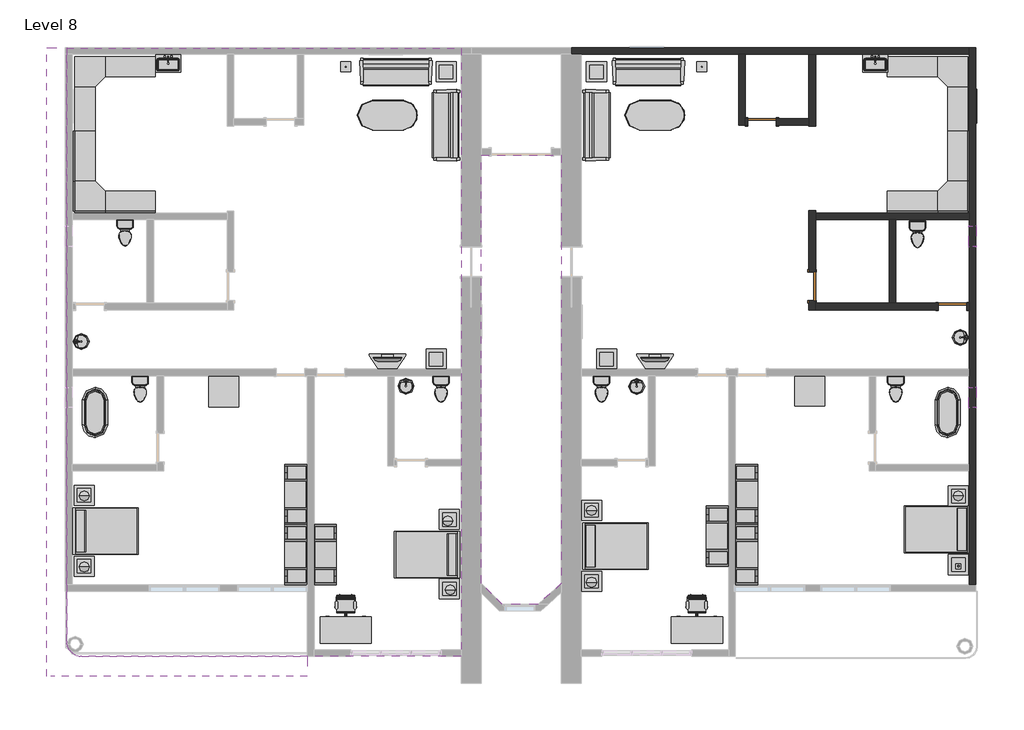
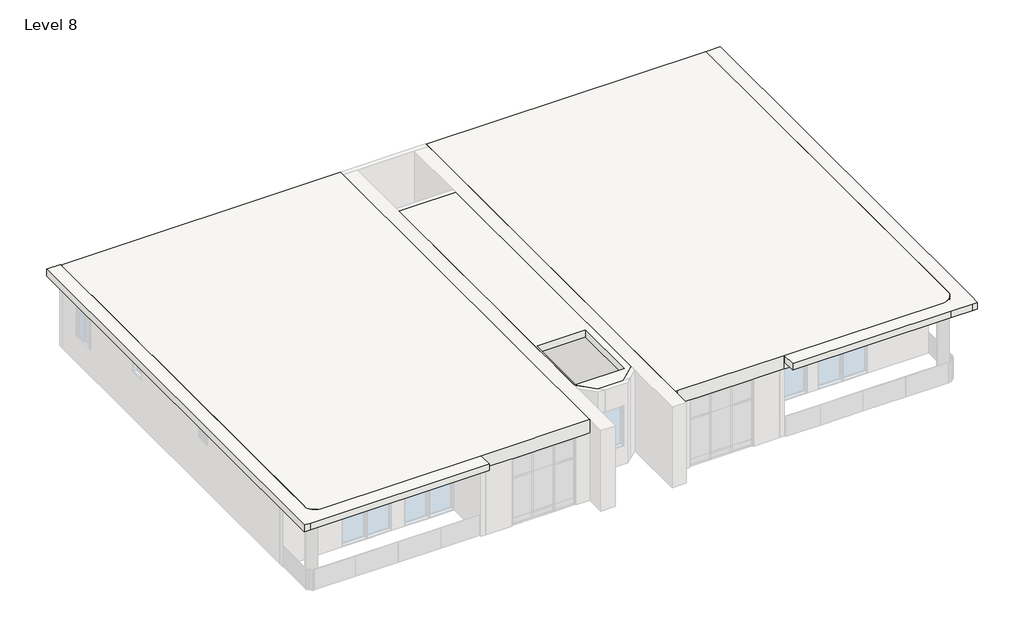
# One storey, part 3 of 3: 42 furniture elements, 14 flow terminals, 10 light fixtures, 9 walls, 3 doors, 3 slabs, 3 windows.
"""IFC4 building model written with IfcOpenShell, lengths in millimetres."""

from ifc_helpers import new_model, si_unit, point, frame, frame_2d, origin, place, context, project, spatial, polyline, circle_curve, trimmed, segment, composite_curve, outline, extrude, faceted_brep, transform, mapped, element, save
from components import door_2703ae13, door_10fd3a06, flow_terminal_38af2918, flow_terminal_d49f872f, toilet_domestic_3d_toilet_domestic_3d_f7549cf7, toilet_domestic_3d_toilet_domestic_3d_183bbd19, flow_terminal_b374fae2, furniture_07436f11, furniture_096e7f55, chair_task_arms_chair_task_arms_fa5a08ef, furniture_072f6425, furniture_cf0b6580, furniture_aff9b2fb, furniture_56245f3a, tv_stand_tv_stand_6ce107e5, furniture_b5c51a22, furniture_2c34a4f9, furniture_4d44e21c, furniture_45e3acac, light_fixture_100w_120v_8564026f, table_lamp_hemispheric_60w_120v_02721d88, window_0038ecf3, window_54100e87

model = new_model("IFC4")

# Units and contexts
model_context = context("Model", 3, world=origin())
ifc_project = project(units=[si_unit("LENGTHUNIT", "METRE", prefix="MILLI")], contexts=[model_context])

# Site, building, storey
site = spatial("IfcSite", under=ifc_project)
building = spatial("IfcBuilding", under=site)
storey = spatial("IfcBuildingStorey", under=building, Name="Level 8", Elevation=25603.2)

# Doors
placement = place(None, origin())
door_shape = door_2703ae13(model_context)
element("IfcDoor", 1, ObjectType="Door-Single-Panel.0001 : 34\" x 80\"", at=placement, inside=storey, context=model_context, shape_type="MappedRepresentation", body=[
    mapped(door_shape, transform((2522.0012296, 9464.0758558, 25603.2), x_axis=(-1.0, 0.0, 0.0), y_axis=(0.0, -1.0, 0.0), z_axis=(0.0, 0.0, 1.0))),
])
door_2_shape = door_10fd3a06(model_context)
element("IfcDoor", 2, ObjectType="Door-Single-Panel.0001 : 34\" x 80\"", at=placement, inside=storey, context=model_context, shape_type="MappedRepresentation", body=[
    mapped(door_2_shape, transform((8313.2012296, 3850.6758558, 25603.2), x_axis=(1.0, 0.0, 0.0), y_axis=(0.0, 1.0, 0.0), z_axis=(0.0, 0.0, 1.0))),
])
element("IfcDoor", 3, ObjectType="Door-Single-Panel.0001 : 34\" x 80\"", at=placement, inside=storey, context=model_context, shape_type="MappedRepresentation", body=[
    mapped(door_2_shape, transform((4046.0012296, 4460.2758558, 25603.2), x_axis=(0.0, -1.0, 0.0), y_axis=(1.0, 0.0, 0.0), z_axis=(0.0, 0.0, 1.0))),
])

# Flow terminals
flow_terminal_shape = flow_terminal_38af2918(model_context)
element("IfcFlowTerminal", 4, ObjectType="Sink Kitchen-Single : 30\" x 21\"", at=placement, inside=storey, context=model_context, shape_type="MappedRepresentation", body=[
    mapped(flow_terminal_shape, transform((-15540.388011, 11239.7304546, 25603.2), x_axis=(1.0, 0.0, 0.0), y_axis=(0.0, 1.0, 0.0), z_axis=(0.0, 0.0, 1.0))),
])
element("IfcFlowTerminal", 5, ObjectType="Sink Kitchen-Single : 30\" x 21\"", at=placement, inside=storey, context=model_context, shape_type="MappedRepresentation", body=[
    mapped(flow_terminal_shape, transform((5948.011989, 11239.7304546, 25603.2), x_axis=(1.0, 0.0, 0.0), y_axis=(0.0, 1.0, 0.0), z_axis=(0.0, 0.0, 1.0))),
])
flow_terminal_2_shape = flow_terminal_d49f872f(model_context)
element("IfcFlowTerminal", 6, ObjectType="Sink Vanity-Round : 19\" x 19\"", at=placement, inside=storey, context=model_context, shape_type="MappedRepresentation", body=[
    mapped(flow_terminal_2_shape, transform((-18084.6070794, 2687.2241152, 25603.2), x_axis=(0.0, 1.0, 0.0), y_axis=(-1.0, 0.0, 0.0), z_axis=(0.0, 0.0, 1.0))),
])
element("IfcFlowTerminal", 7, ObjectType="Sink Vanity-Round : 19\" x 19\"", at=placement, inside=storey, context=model_context, shape_type="MappedRepresentation", body=[
    mapped(flow_terminal_2_shape, transform((8462.2249463, 3007.5275963, 25603.2), x_axis=(0.0, -1.0, 0.0), y_axis=(1.0, 0.0, 0.0), z_axis=(0.0, 0.0, 1.0))),
])
element("IfcFlowTerminal", 8, ObjectType="Sink Vanity-Round : 19\" x 19\"", at=placement, inside=storey, context=model_context, shape_type="MappedRepresentation", body=[
    mapped(flow_terminal_2_shape, transform((-8395.050511, 1341.8921141, 25603.2), x_axis=(1.0, 0.0, 0.0), y_axis=(0.0, 1.0, 0.0), z_axis=(0.0, 0.0, 1.0))),
])
element("IfcFlowTerminal", 9, ObjectType="Sink Vanity-Round : 19\" x 19\"", at=placement, inside=storey, context=model_context, shape_type="MappedRepresentation", body=[
    mapped(flow_terminal_2_shape, transform((-1384.650511, 1331.0855344, 25603.2), x_axis=(1.0, 0.0, 0.0), y_axis=(0.0, 1.0, 0.0), z_axis=(0.0, 0.0, 1.0))),
])
toilet_domestic_3d_toilet_domestic_3d_shape = toilet_domestic_3d_toilet_domestic_3d_f7549cf7(model_context)
toilet_domestic_3d_toilet_domestic_3d_2_shape = toilet_domestic_3d_toilet_domestic_3d_183bbd19(model_context)
element("IfcFlowTerminal", 10, ObjectType="Toilet-Domestic-3D : Toilet-Domestic-3D", at=placement, inside=storey, context=model_context, shape_type="MappedRepresentation", body=[
    mapped(toilet_domestic_3d_toilet_domestic_3d_shape, transform((6586.0012296, 1247.7798284, 25603.2), x_axis=(1.0, 0.0, 0.0), y_axis=(0.0, 1.0, 0.0), z_axis=(0.0, 0.0, 1.0))),
    mapped(toilet_domestic_3d_toilet_domestic_3d_2_shape, transform((6586.0012296, 1247.7798284, 25603.2), x_axis=(1.0, 0.0, 0.0), y_axis=(0.0, 1.0, 0.0), z_axis=(0.0, 0.0, 1.0))),
])
element("IfcFlowTerminal", 11, ObjectType="Toilet-Domestic-3D : Toilet-Domestic-3D", at=placement, inside=storey, context=model_context, shape_type="MappedRepresentation", body=[
    mapped(toilet_domestic_3d_toilet_domestic_3d_shape, transform((-2354.7987704, 1247.7798284, 25603.2), x_axis=(1.0, 0.0, 0.0), y_axis=(0.0, 1.0, 0.0), z_axis=(0.0, 0.0, 1.0))),
    mapped(toilet_domestic_3d_toilet_domestic_3d_2_shape, transform((-2354.7987704, 1247.7798284, 25603.2), x_axis=(1.0, 0.0, 0.0), y_axis=(0.0, 1.0, 0.0), z_axis=(0.0, 0.0, 1.0))),
])
element("IfcFlowTerminal", 12, ObjectType="Toilet-Domestic-3D : Toilet-Domestic-3D", at=placement, inside=storey, context=model_context, shape_type="MappedRepresentation", body=[
    mapped(toilet_domestic_3d_toilet_domestic_3d_shape, transform((-16375.5987704, 1247.7798284, 25603.2), x_axis=(1.0, 0.0, 0.0), y_axis=(0.0, 1.0, 0.0), z_axis=(0.0, 0.0, 1.0))),
    mapped(toilet_domestic_3d_toilet_domestic_3d_2_shape, transform((-16375.5987704, 1247.7798284, 25603.2), x_axis=(1.0, 0.0, 0.0), y_axis=(0.0, 1.0, 0.0), z_axis=(0.0, 0.0, 1.0))),
])
element("IfcFlowTerminal", 13, ObjectType="Toilet-Domestic-3D : Toilet-Domestic-3D", at=placement, inside=storey, context=model_context, shape_type="MappedRepresentation", body=[
    mapped(toilet_domestic_3d_toilet_domestic_3d_shape, transform((-16832.7987704, 5997.5798284, 25603.2), x_axis=(1.0, 0.0, 0.0), y_axis=(0.0, 1.0, 0.0), z_axis=(0.0, 0.0, 1.0))),
    mapped(toilet_domestic_3d_toilet_domestic_3d_2_shape, transform((-16832.7987704, 5997.5798284, 25603.2), x_axis=(1.0, 0.0, 0.0), y_axis=(0.0, 1.0, 0.0), z_axis=(0.0, 0.0, 1.0))),
])
element("IfcFlowTerminal", 14, ObjectType="Toilet-Domestic-3D : Toilet-Domestic-3D", at=placement, inside=storey, context=model_context, shape_type="MappedRepresentation", body=[
    mapped(toilet_domestic_3d_toilet_domestic_3d_shape, transform((7246.4012296, 5946.7798284, 25603.2), x_axis=(1.0, 0.0, 0.0), y_axis=(0.0, 1.0, 0.0), z_axis=(0.0, 0.0, 1.0))),
    mapped(toilet_domestic_3d_toilet_domestic_3d_2_shape, transform((7246.4012296, 5946.7798284, 25603.2), x_axis=(1.0, 0.0, 0.0), y_axis=(0.0, 1.0, 0.0), z_axis=(0.0, 0.0, 1.0))),
])
element("IfcFlowTerminal", 15, ObjectType="Toilet-Domestic-3D : Toilet-Domestic-3D", at=placement, inside=storey, context=model_context, shape_type="MappedRepresentation", body=[
    mapped(toilet_domestic_3d_toilet_domestic_3d_shape, transform((-7231.5987704, 1247.7798284, 25603.2), x_axis=(1.0, 0.0, 0.0), y_axis=(0.0, 1.0, 0.0), z_axis=(0.0, 0.0, 1.0))),
    mapped(toilet_domestic_3d_toilet_domestic_3d_2_shape, transform((-7231.5987704, 1247.7798284, 25603.2), x_axis=(1.0, 0.0, 0.0), y_axis=(0.0, 1.0, 0.0), z_axis=(0.0, 0.0, 1.0))),
])
flow_terminal_3_shape = flow_terminal_b374fae2(model_context)
element("IfcFlowTerminal", 16, ObjectType="Tub-Free Standing-3D : 30\" x 60\"", at=placement, inside=storey, context=model_context, shape_type="MappedRepresentation", body=[
    mapped(flow_terminal_3_shape, transform((-17747.1987704, 624.8758558, 25603.2), x_axis=(1.0, 0.0, 0.0), y_axis=(0.0, 1.0, 0.0), z_axis=(0.0, 0.0, 1.0))),
])
element("IfcFlowTerminal", 17, ObjectType="Tub-Free Standing-3D : 30\" x 60\"", at=placement, inside=storey, context=model_context, shape_type="MappedRepresentation", body=[
    mapped(flow_terminal_3_shape, transform((8160.8012296, 624.8758558, 25603.2), x_axis=(1.0, 0.0, 0.0), y_axis=(0.0, 1.0, 0.0), z_axis=(0.0, 0.0, 1.0))),
])

# Furniture
furniture_shape = furniture_07436f11(model_context)
element("IfcFurniture", 18, ObjectType="96\" x 96\"", at=placement, inside=storey, context=model_context, shape_type="MappedRepresentation", body=[
    mapped(furniture_shape, transform((-18275.8670182, 11991.0988634, 25603.2), x_axis=(1.0, 0.0, 0.0), y_axis=(0.0, 1.0, 0.0), z_axis=(0.0, 0.0, 1.0))),
])
element("IfcFurniture", 19, ObjectType="96\" x 96\"", at=placement, inside=storey, context=model_context, shape_type="MappedRepresentation", body=[
    mapped(furniture_shape, transform((9316.2242372, 11364.3441035, 25603.2), x_axis=(0.0, -1.0, 0.0), y_axis=(1.0, 0.0, 0.0), z_axis=(0.0, 0.0, 1.0))),
])
furniture_2_shape = furniture_096e7f55(model_context)
element("IfcFurniture", 20, ObjectType="Bed-Shaker : Double 56\" x 78\"", at=placement, inside=storey, context=model_context, shape_type="MappedRepresentation", body=[
    mapped(furniture_2_shape, transform((-18407.5987704, -2962.8741442, 25603.2), x_axis=(0.0, 1.0, 0.0), y_axis=(-1.0, 0.0, 0.0), z_axis=(0.0, 0.0, 1.0))),
])
element("IfcFurniture", 21, ObjectType="Bed-Shaker : Double 56\" x 78\"", at=placement, inside=storey, context=model_context, shape_type="MappedRepresentation", body=[
    mapped(furniture_2_shape, transform((-6672.7987704, -3712.1741442, 25603.2), x_axis=(0.0, -1.0, 0.0), y_axis=(1.0, 0.0, 0.0), z_axis=(0.0, 0.0, 1.0))),
])
element("IfcFurniture", 22, ObjectType="Bed-Shaker : Double 56\" x 78\"", at=placement, inside=storey, context=model_context, shape_type="MappedRepresentation", body=[
    mapped(furniture_2_shape, transform((-2913.5987704, -3420.0741442, 25603.2), x_axis=(0.0, 1.0, 0.0), y_axis=(-1.0, 0.0, 0.0), z_axis=(0.0, 0.0, 1.0))),
])
element("IfcFurniture", 23, ObjectType="Bed-Shaker : Double 56\" x 78\"", at=placement, inside=storey, context=model_context, shape_type="MappedRepresentation", body=[
    mapped(furniture_2_shape, transform((8821.2012296, -2950.1741442, 25603.2), x_axis=(0.0, -1.0, 0.0), y_axis=(1.0, 0.0, 0.0), z_axis=(0.0, 0.0, 1.0))),
])
chair_task_arms_chair_task_arms_shape = chair_task_arms_chair_task_arms_fa5a08ef(model_context)
element("IfcFurniture", 24, ObjectType="Chair-Task Arms : Chair-Task Arms", at=placement, inside=storey, context=model_context, shape_type="MappedRepresentation", body=[
    mapped(chair_task_arms_chair_task_arms_shape, transform((681.7920493, -5184.3566833, 25603.2), x_axis=(-1.0, 0.0, 0.0), y_axis=(0.0, -1.0, 0.0), z_axis=(0.0, 0.0, 1.0))),
])
element("IfcFurniture", 25, ObjectType="Chair-Task Arms : Chair-Task Arms", at=placement, inside=storey, context=model_context, shape_type="MappedRepresentation", body=[
    mapped(chair_task_arms_chair_task_arms_shape, transform((-9986.2079507, -5184.3566833, 25603.2), x_axis=(-1.0, 0.0, 0.0), y_axis=(0.0, -1.0, 0.0), z_axis=(0.0, 0.0, 1.0))),
])
furniture_3_shape = furniture_072f6425(model_context)
element("IfcFurniture", 26, ObjectType="Desk : 60\" x 30\"", at=placement, inside=storey, context=model_context, shape_type="MappedRepresentation", body=[
    mapped(furniture_3_shape, transform((-10889.1987704, -6371.702585, 25603.2), x_axis=(1.0, 0.0, 0.0), y_axis=(0.0, 1.0, 0.0), z_axis=(0.0, 0.0, 1.0))),
])
element("IfcFurniture", 27, ObjectType="Desk : 60\" x 30\"", at=placement, inside=storey, context=model_context, shape_type="MappedRepresentation", body=[
    mapped(furniture_3_shape, transform((-221.1987704, -6371.702585, 25603.2), x_axis=(1.0, 0.0, 0.0), y_axis=(0.0, 1.0, 0.0), z_axis=(0.0, 0.0, 1.0))),
])
furniture_4_shape = furniture_cf0b6580(model_context)
element("IfcFurniture", 28, ObjectType="Entertainment Center : 72\" x 72\" x 24\"", at=placement, inside=storey, context=model_context, shape_type="MappedRepresentation", body=[
    mapped(furniture_4_shape, transform((1607.6012296, -3134.3241442, 25603.2), x_axis=(0.0, -1.0, 0.0), y_axis=(1.0, 0.0, 0.0), z_axis=(0.0, 0.0, 1.0))),
])
element("IfcFurniture", 29, ObjectType="Entertainment Center : 72\" x 72\" x 24\"", at=placement, inside=storey, context=model_context, shape_type="MappedRepresentation", body=[
    mapped(furniture_4_shape, transform((1607.6012296, -3693.1241442, 25603.2), x_axis=(0.0, 1.0, 0.0), y_axis=(-1.0, 0.0, 0.0), z_axis=(0.0, 0.0, 1.0))),
])
element("IfcFurniture", 30, ObjectType="Entertainment Center : 72\" x 72\" x 24\"", at=placement, inside=storey, context=model_context, shape_type="MappedRepresentation", body=[
    mapped(furniture_4_shape, transform((1607.6012296, -1864.3241442, 25603.2), x_axis=(0.0, 1.0, 0.0), y_axis=(-1.0, 0.0, 0.0), z_axis=(0.0, 0.0, 1.0))),
])
element("IfcFurniture", 31, ObjectType="Entertainment Center : 72\" x 72\" x 24\"", at=placement, inside=storey, context=model_context, shape_type="MappedRepresentation", body=[
    mapped(furniture_4_shape, transform((-11193.9987704, -3693.1241442, 25603.2), x_axis=(0.0, -1.0, 0.0), y_axis=(1.0, 0.0, 0.0), z_axis=(0.0, 0.0, 1.0))),
])
element("IfcFurniture", 32, ObjectType="Entertainment Center : 72\" x 72\" x 24\"", at=placement, inside=storey, context=model_context, shape_type="MappedRepresentation", body=[
    mapped(furniture_4_shape, transform((-11193.9987704, -1864.3241442, 25603.2), x_axis=(0.0, -1.0, 0.0), y_axis=(1.0, 0.0, 0.0), z_axis=(0.0, 0.0, 1.0))),
])
element("IfcFurniture", 33, ObjectType="Entertainment Center : 72\" x 72\" x 24\"", at=placement, inside=storey, context=model_context, shape_type="MappedRepresentation", body=[
    mapped(furniture_4_shape, transform((-11193.9987704, -3693.1241442, 25603.2), x_axis=(0.0, 1.0, 0.0), y_axis=(-1.0, 0.0, 0.0), z_axis=(0.0, 0.0, 1.0))),
])
furniture_5_shape = furniture_aff9b2fb(model_context)
element("IfcFurniture", 34, ObjectType="Sofa-Pensi : 84\"", at=placement, inside=storey, context=model_context, shape_type="MappedRepresentation", body=[
    mapped(furniture_5_shape, transform((-8881.8050204, 10710.9660197, 25603.2), x_axis=(1.0, 0.0, 0.0), y_axis=(0.0, 1.0, 0.0), z_axis=(0.0, 0.0, 1.0))),
])
element("IfcFurniture", 35, ObjectType="Sofa-Pensi : 84\"", at=placement, inside=storey, context=model_context, shape_type="MappedRepresentation", body=[
    mapped(furniture_5_shape, transform((-7356.3086065, 9641.0821058, 25603.2), x_axis=(0.0, -1.0, 0.0), y_axis=(1.0, 0.0, 0.0), z_axis=(0.0, 0.0, 1.0))),
])
element("IfcFurniture", 36, ObjectType="Sofa-Pensi : 84\"", at=placement, inside=storey, context=model_context, shape_type="MappedRepresentation", body=[
    mapped(furniture_5_shape, transform((-2230.0889343, 9083.8696058, 25603.2), x_axis=(0.0, 1.0, 0.0), y_axis=(-1.0, 0.0, 0.0), z_axis=(0.0, 0.0, 1.0))),
])
element("IfcFurniture", 37, ObjectType="Sofa-Pensi : 84\"", at=placement, inside=storey, context=model_context, shape_type="MappedRepresentation", body=[
    mapped(furniture_5_shape, transform((-1211.0050204, 10710.9660197, 25603.2), x_axis=(1.0, 0.0, 0.0), y_axis=(0.0, 1.0, 0.0), z_axis=(0.0, 0.0, 1.0))),
])
furniture_6_shape = furniture_56245f3a(model_context)
element("IfcFurniture", 38, ObjectType="TV - Flat Screen : 32\"", at=placement, inside=storey, context=model_context, shape_type="MappedRepresentation", body=[
    mapped(furniture_6_shape, transform((-8861.1432846, 2232.8144794, 26517.6), x_axis=(-1.0, 0.0, 0.0), y_axis=(0.0, -1.0, 0.0), z_axis=(0.0, 0.0, 1.0))),
])
element("IfcFurniture", 39, ObjectType="TV - Flat Screen : 32\"", at=placement, inside=storey, context=model_context, shape_type="MappedRepresentation", body=[
    mapped(furniture_6_shape, transform((-733.1432846, 2232.8144794, 26517.6), x_axis=(-1.0, 0.0, 0.0), y_axis=(0.0, -1.0, 0.0), z_axis=(0.0, 0.0, 1.0))),
])
tv_stand_tv_stand_shape = tv_stand_tv_stand_6ce107e5(model_context)
element("IfcFurniture", 40, ObjectType="TV Stand : TV Stand", at=placement, inside=storey, context=model_context, shape_type="MappedRepresentation", body=[
    mapped(tv_stand_tv_stand_shape, transform((-8732.0107683, 1945.6758558, 25603.2), x_axis=(-1.0, 0.0, 0.0), y_axis=(0.0, -1.0, 0.0), z_axis=(0.0, 0.0, 1.0))),
])
element("IfcFurniture", 41, ObjectType="TV Stand : TV Stand", at=placement, inside=storey, context=model_context, shape_type="MappedRepresentation", body=[
    mapped(tv_stand_tv_stand_shape, transform((-604.0107683, 1945.6758558, 25603.2), x_axis=(-1.0, 0.0, 0.0), y_axis=(0.0, -1.0, 0.0), z_axis=(0.0, 0.0, 1.0))),
])
furniture_7_shape = furniture_b5c51a22(model_context)
element("IfcFurniture", 42, ObjectType="Table-Coffee : 24\" x 24\" x 24\"", at=placement, inside=storey, context=model_context, shape_type="MappedRepresentation", body=[
    mapped(furniture_7_shape, transform((-7097.4645371, 10892.864778, 25603.2), x_axis=(1.0, 0.0, 0.0), y_axis=(0.0, 1.0, 0.0), z_axis=(0.0, 0.0, 1.0))),
])
element("IfcFurniture", 43, ObjectType="Table-Coffee : 24\" x 24\" x 24\"", at=placement, inside=storey, context=model_context, shape_type="MappedRepresentation", body=[
    mapped(furniture_7_shape, transform((-2525.4645371, 10892.864778, 25603.2), x_axis=(1.0, 0.0, 0.0), y_axis=(0.0, 1.0, 0.0), z_axis=(0.0, 0.0, 1.0))),
])
element("IfcFurniture", 44, ObjectType="Table-Coffee : 24\" x 24\" x 24\"", at=placement, inside=storey, context=model_context, shape_type="MappedRepresentation", body=[
    mapped(furniture_7_shape, transform((-7402.2645371, 2155.264778, 25603.2), x_axis=(1.0, 0.0, 0.0), y_axis=(0.0, 1.0, 0.0), z_axis=(0.0, 0.0, 1.0))),
])
element("IfcFurniture", 45, ObjectType="Table-Coffee : 24\" x 24\" x 24\"", at=placement, inside=storey, context=model_context, shape_type="MappedRepresentation", body=[
    mapped(furniture_7_shape, transform((-2220.6645371, 2155.264778, 25603.2), x_axis=(1.0, 0.0, 0.0), y_axis=(0.0, 1.0, 0.0), z_axis=(0.0, 0.0, 1.0))),
])
element("IfcFurniture", 46, ObjectType="Table-Coffee : 24\" x 24\" x 24\"", at=placement, inside=storey, context=model_context, shape_type="MappedRepresentation", body=[
    mapped(furniture_7_shape, transform((-2677.8645371, -4601.135222, 25603.2), x_axis=(1.0, 0.0, 0.0), y_axis=(0.0, 1.0, 0.0), z_axis=(0.0, 0.0, 1.0))),
])
element("IfcFurniture", 47, ObjectType="Table-Coffee : 24\" x 24\" x 24\"", at=placement, inside=storey, context=model_context, shape_type="MappedRepresentation", body=[
    mapped(furniture_7_shape, transform((-18095.6645371, -4143.935222, 25603.2), x_axis=(1.0, 0.0, 0.0), y_axis=(0.0, 1.0, 0.0), z_axis=(0.0, 0.0, 1.0))),
])
element("IfcFurniture", 48, ObjectType="Table-Coffee : 24\" x 24\" x 24\"", at=placement, inside=storey, context=model_context, shape_type="MappedRepresentation", body=[
    mapped(furniture_7_shape, transform((-18095.6645371, -1984.935222, 25603.2), x_axis=(1.0, 0.0, 0.0), y_axis=(0.0, 1.0, 0.0), z_axis=(0.0, 0.0, 1.0))),
])
element("IfcFurniture", 49, ObjectType="Table-Coffee : 24\" x 24\" x 24\"", at=placement, inside=storey, context=model_context, shape_type="MappedRepresentation", body=[
    mapped(furniture_7_shape, transform((-2677.8645371, -2442.135222, 25603.2), x_axis=(1.0, 0.0, 0.0), y_axis=(0.0, 1.0, 0.0), z_axis=(0.0, 0.0, 1.0))),
])
element("IfcFurniture", 50, ObjectType="Table-Coffee : 24\" x 24\" x 24\"", at=placement, inside=storey, context=model_context, shape_type="MappedRepresentation", body=[
    mapped(furniture_7_shape, transform((8472.7354629, -4093.135222, 25603.2), x_axis=(1.0, 0.0, 0.0), y_axis=(0.0, 1.0, 0.0), z_axis=(0.0, 0.0, 1.0))),
])
element("IfcFurniture", 51, ObjectType="Table-Coffee : 24\" x 24\" x 24\"", at=placement, inside=storey, context=model_context, shape_type="MappedRepresentation", body=[
    mapped(furniture_7_shape, transform((8472.7354629, -2010.335222, 25603.2), x_axis=(1.0, 0.0, 0.0), y_axis=(0.0, 1.0, 0.0), z_axis=(0.0, 0.0, 1.0))),
])
element("IfcFurniture", 52, ObjectType="Table-Coffee : 24\" x 24\" x 24\"", at=placement, inside=storey, context=model_context, shape_type="MappedRepresentation", body=[
    mapped(furniture_7_shape, transform((-6995.8645371, -4832.0414601, 25603.2), x_axis=(1.0, 0.0, 0.0), y_axis=(0.0, 1.0, 0.0), z_axis=(0.0, 0.0, 1.0))),
])
element("IfcFurniture", 53, ObjectType="Table-Coffee : 24\" x 24\" x 24\"", at=placement, inside=storey, context=model_context, shape_type="MappedRepresentation", body=[
    mapped(furniture_7_shape, transform((-6995.8645371, -2723.8414601, 25603.2), x_axis=(1.0, 0.0, 0.0), y_axis=(0.0, 1.0, 0.0), z_axis=(0.0, 0.0, 1.0))),
])
furniture_8_shape = furniture_2c34a4f9(model_context)
element("IfcFurniture", 54, ObjectType="Table-Dining Oval : 36\" x 72\"", at=placement, inside=storey, context=model_context, shape_type="MappedRepresentation", body=[
    mapped(furniture_8_shape, transform((-8455.3790983, 10025.3742164, 25603.2), x_axis=(1.0, 0.0, 0.0), y_axis=(0.0, 1.0, 0.0), z_axis=(0.0, 0.0, 1.0))),
])
element("IfcFurniture", 55, ObjectType="Table-Dining Oval : 36\" x 72\"", at=placement, inside=storey, context=model_context, shape_type="MappedRepresentation", body=[
    mapped(furniture_8_shape, transform((-327.3790983, 10025.3742164, 25603.2), x_axis=(1.0, 0.0, 0.0), y_axis=(0.0, 1.0, 0.0), z_axis=(0.0, 0.0, 1.0))),
])
furniture_9_shape = furniture_4d44e21c(model_context)
element("IfcFurniture", 56, ObjectType="Table-Rectangular : 36\" x 36\"", at=placement, inside=storey, context=model_context, shape_type="MappedRepresentation", body=[
    mapped(furniture_9_shape, transform((-13835.5987704, 1259.8758558, 25603.2), x_axis=(1.0, 0.0, 0.0), y_axis=(0.0, 1.0, 0.0), z_axis=(0.0, 0.0, 1.0))),
])
element("IfcFurniture", 57, ObjectType="Table-Rectangular : 36\" x 36\"", at=placement, inside=storey, context=model_context, shape_type="MappedRepresentation", body=[
    mapped(furniture_9_shape, transform((3969.8012296, 1285.2758558, 25603.2), x_axis=(1.0, 0.0, 0.0), y_axis=(0.0, 1.0, 0.0), z_axis=(0.0, 0.0, 1.0))),
])
furniture_10_shape = furniture_45e3acac(model_context)
element("IfcFurniture", 58, ObjectType="Work Station Cubicle : 96\" x 96\"", at=placement, inside=storey, context=model_context, shape_type="MappedRepresentation", body=[
    mapped(furniture_10_shape, transform((-18902.621778, 6827.207608, 25603.2), x_axis=(0.0, 1.0, 0.0), y_axis=(-1.0, 0.0, 0.0), z_axis=(0.0, 0.0, 1.0))),
])
element("IfcFurniture", 59, ObjectType="Work Station Cubicle : 96\" x 96\"", at=placement, inside=storey, context=model_context, shape_type="MappedRepresentation", body=[
    mapped(furniture_10_shape, transform((8689.4694774, 6200.4528481, 25603.2), x_axis=(-1.0, 0.0, 0.0), y_axis=(0.0, -1.0, 0.0), z_axis=(0.0, 0.0, 1.0))),
])

# Light fixtures
light_fixture_100w_120v_shape = light_fixture_100w_120v_8564026f(model_context)
element("IfcLightFixture", 60, ObjectType="100W - 120V", at=placement, inside=storey, context=model_context, shape_type="MappedRepresentation", body=[
    mapped(light_fixture_100w_120v_shape, transform((-10127.1987704, 11140.4758558, 25603.2), x_axis=(1.0, 0.0, 0.0), y_axis=(0.0, 1.0, 0.0), z_axis=(0.0, 0.0, 1.0))),
])
element("IfcLightFixture", 61, ObjectType="100W - 120V", at=placement, inside=storey, context=model_context, shape_type="MappedRepresentation", body=[
    mapped(light_fixture_100w_120v_shape, transform((693.2012296, 11140.4758558, 25603.2), x_axis=(1.0, 0.0, 0.0), y_axis=(0.0, 1.0, 0.0), z_axis=(0.0, 0.0, 1.0))),
])
table_lamp_hemispheric_60w_120v_shape = table_lamp_hemispheric_60w_120v_02721d88(model_context)
element("IfcLightFixture", 62, ObjectType="Table Lamp - Hemispheric : 60W - 120V", at=placement, inside=storey, context=model_context, shape_type="MappedRepresentation", body=[
    mapped(table_lamp_hemispheric_60w_120v_shape, transform((-18077.3987704, -1915.1241442, 26212.8), x_axis=(1.0, 0.0, 0.0), y_axis=(0.0, 1.0, 0.0), z_axis=(0.0, 0.0, 1.0))),
])
element("IfcLightFixture", 63, ObjectType="Table Lamp - Hemispheric : 60W - 120V", at=placement, inside=storey, context=model_context, shape_type="MappedRepresentation", body=[
    mapped(table_lamp_hemispheric_60w_120v_shape, transform((-7028.3987704, -2666.7303823, 26212.8), x_axis=(1.0, 0.0, 0.0), y_axis=(0.0, 1.0, 0.0), z_axis=(0.0, 0.0, 1.0))),
])
element("IfcLightFixture", 64, ObjectType="Table Lamp - Hemispheric : 60W - 120V", at=placement, inside=storey, context=model_context, shape_type="MappedRepresentation", body=[
    mapped(table_lamp_hemispheric_60w_120v_shape, transform((-2659.5987704, -2346.9241442, 26212.8), x_axis=(1.0, 0.0, 0.0), y_axis=(0.0, 1.0, 0.0), z_axis=(0.0, 0.0, 1.0))),
])
element("IfcLightFixture", 65, ObjectType="Table Lamp - Hemispheric : 60W - 120V", at=placement, inside=storey, context=model_context, shape_type="MappedRepresentation", body=[
    mapped(table_lamp_hemispheric_60w_120v_shape, transform((8491.0012296, -4048.7241442, 26517.6), x_axis=(1.0, 0.0, 0.0), y_axis=(0.0, 1.0, 0.0), z_axis=(0.0, 0.0, 1.0))),
])
element("IfcLightFixture", 66, ObjectType="Table Lamp - Hemispheric : 60W - 120V", at=placement, inside=storey, context=model_context, shape_type="MappedRepresentation", body=[
    mapped(table_lamp_hemispheric_60w_120v_shape, transform((8491.0012296, -1915.1241442, 26212.8), x_axis=(1.0, 0.0, 0.0), y_axis=(0.0, 1.0, 0.0), z_axis=(0.0, 0.0, 1.0))),
])
element("IfcLightFixture", 67, ObjectType="Table Lamp - Hemispheric : 60W - 120V", at=placement, inside=storey, context=model_context, shape_type="MappedRepresentation", body=[
    mapped(table_lamp_hemispheric_60w_120v_shape, transform((-2659.5987704, -4531.3241442, 26212.8), x_axis=(1.0, 0.0, 0.0), y_axis=(0.0, 1.0, 0.0), z_axis=(0.0, 0.0, 1.0))),
])
element("IfcLightFixture", 68, ObjectType="Table Lamp - Hemispheric : 60W - 120V", at=placement, inside=storey, context=model_context, shape_type="MappedRepresentation", body=[
    mapped(table_lamp_hemispheric_60w_120v_shape, transform((-6952.1987704, -4762.2303823, 26212.8), x_axis=(1.0, 0.0, 0.0), y_axis=(0.0, 1.0, 0.0), z_axis=(0.0, 0.0, 1.0))),
])
element("IfcLightFixture", 69, ObjectType="Table Lamp - Hemispheric : 60W - 120V", at=placement, inside=storey, context=model_context, shape_type="MappedRepresentation", body=[
    mapped(table_lamp_hemispheric_60w_120v_shape, transform((-18077.3987704, -4074.1241442, 26212.8), x_axis=(1.0, 0.0, 0.0), y_axis=(0.0, 1.0, 0.0), z_axis=(0.0, 0.0, 1.0))),
])

# Slabs
element("IfcSlab", 70, ObjectType="Generic - 12\" cream", at=placement, inside=storey, context=model_context, shape_type="SweptSolid", body=[
    extrude(outline(composite_curve([segment(polyline([(-6621.9987704, 11699.2758558), (-6621.9987704, -6791.9241442), (-11295.5987704, -6791.9241442), (-18153.5987704, -6791.9241442)]), True, "CONTINUOUS"), segment(trimmed(circle_curve(frame_2d((-18153.5987704, -6334.7241442)), 457.2), [point((-18153.5987704, -6791.9241442))], [point((-18610.7987704, -6334.7241442))], False, "CARTESIAN"), True, "CONTINUOUS"), segment(polyline([(-18610.7987704, -6334.7241442), (-18610.7987704, 11699.2758558), (-6621.9987704, 11699.2758558)]), True, "CONTINUOUS")], self_intersect=False)), frame((0.0, 0.0, 28651.2), z_axis=(0.0, 0.0, 1.0), x_axis=(1.0, 0.0, 0.0)), (0.0, 0.0, 1.0), 609.6),
    extrude(outline(composite_curve([segment(trimmed(circle_curve(frame_2d((8511.8043381, -6277.3874522)), 514.536692), [point((9024.4012296, -6322.0241442))], [point((8511.8043381, -6791.9241442))], False, "CARTESIAN"), True, "CONTINUOUS"), segment(polyline([(8511.8043381, -6791.9241442), (1709.2012296, -6791.9241442), (-2862.7987704, -6791.9241442), (-2964.3987704, -6791.9241442), (-2964.3987704, 11699.2758558), (9024.4012296, 11699.2758558), (9024.4012296, -6322.0241442)]), True, "CONTINUOUS")], self_intersect=False)), frame((0.0, 0.0, 28651.2), z_axis=(0.0, 0.0, 1.0), x_axis=(1.0, 0.0, 0.0)), (0.0, 0.0, 1.0), 609.6),
])
element("IfcSlab", 71, ObjectType="Generic - 12\" white", at=placement, inside=storey, context=model_context, shape_type="SweptSolid", body=[
    extrude(outline(composite_curve([segment(polyline([(9634.0012296, 11699.2758558), (9634.0012296, -6931.6241442), (9634.0012296, -7401.5241442), (9430.8012296, -7401.5241442), (8511.8043381, -7401.5241442), (1709.2012296, -7401.5241442), (1709.2012296, -6791.9241442), (8511.8043381, -6791.9241442)]), True, "CONTINUOUS"), segment(trimmed(circle_curve(frame_2d((8511.8043381, -6277.3874522)), 514.536692), [point((8511.8043381, -6791.9241442))], [point((9024.4012296, -6322.0241442))], True, "CARTESIAN"), True, "CONTINUOUS"), segment(polyline([(9024.4012296, -6322.0241442), (9024.4012296, 11699.2758558), (9634.0012296, 11699.2758558)]), True, "CONTINUOUS")], self_intersect=False)), frame((0.0, 0.0, 28956.0), z_axis=(0.0, 0.0, 1.0), x_axis=(1.0, 0.0, 0.0)), (0.0, 0.0, 1.0), 304.8),
    extrude(outline(composite_curve([segment(polyline([(-18610.7987704, 11724.6758558), (-18610.7987704, -6334.7241442)]), True, "CONTINUOUS"), segment(trimmed(circle_curve(frame_2d((-18153.5987704, -6334.7241442)), 457.2), [point((-18610.7987704, -6334.7241442))], [point((-18153.5987704, -6791.9241442))], True, "CARTESIAN"), True, "CONTINUOUS"), segment(polyline([(-18153.5987704, -6791.9241442), (-11295.5987704, -6791.9241442), (-11295.5987704, -7401.5241442), (-18966.3987704, -7401.5241442), (-19220.3987704, -7401.5241442), (-19220.3987704, 11724.6758558), (-18610.7987704, 11724.6758558)]), True, "CONTINUOUS")], self_intersect=False)), frame((0.0, 0.0, 28956.0), z_axis=(0.0, 0.0, 1.0), x_axis=(1.0, 0.0, 0.0)), (0.0, 0.0, 1.0), 304.8),
])
element("IfcSlab", 72, ObjectType="Generic - 12\" white", at=placement, inside=storey, context=model_context, shape_type="SweptSolid", body=[
    extrude(outline(polyline([(-3573.9987704, 8448.0758558), (-3573.9987704, -1691.5549149), (-3573.9987704, -4572.9908503), (-4280.7801413, -5203.302585), (-5374.5362318, -5203.302585), (-6012.3987704, -4565.4400463), (-6012.3987704, -1691.5549149), (-6012.3987704, 8448.0758558), (-3573.9987704, 8448.0758558)]), holes=[polyline([(-5940.8822214, -4561.7549149), (-3870.7822214, -4561.7549149), (-3870.7822214, -1691.5549149), (-5940.8822214, -1691.5549149), (-5940.8822214, -4561.7549149)])]), frame((0.0, 0.0, 28956.0), z_axis=(0.0, 0.0, 1.0), x_axis=(1.0, 0.0, 0.0)), (0.0, 0.0, 1.0), 304.8),
])

# Walls
element("IfcWall", 73, ObjectType="Generic - 8\" cream", at=placement, inside=storey, context=model_context, shape_type="Brep", body=[
    faceted_brep([(8821.2012296, 11724.6758558, 25603.2), (8821.2012296, 11521.4758558, 25603.2), (8821.2012296, 6695.4758558, 25603.2), (8821.2012296, 6492.2758558, 25603.2), (8821.2012296, 3952.2758558, 25603.2), (8821.2012296, 3749.0758558, 25603.2), (8821.2012296, 1945.6758558, 25603.2), (8821.2012296, 1742.4758558, 25603.2), (8821.2012296, -949.9241442, 25603.2), (8821.2012296, -1153.1241442, 25603.2), (8821.2012296, -4607.5241442, 25603.2), (8821.2012296, -4607.5241442, 28651.2), (8821.2012296, -1153.1241442, 28651.2), (8821.2012296, -949.9241442, 28651.2), (8821.2012296, 1742.4758558, 28651.2), (8821.2012296, 1945.6758558, 28651.2), (8821.2012296, 3749.0758558, 28651.2), (8821.2012296, 3952.2758558, 28651.2), (8821.2012296, 6492.2758558, 28651.2), (8821.2012296, 6695.4758558, 28651.2), (8821.2012296, 11521.4758558, 28651.2), (8821.2012296, 11724.6758558, 28651.2), (8821.2012296, 10403.8758558, 26822.4), (8821.2012296, 10403.8758558, 28041.6), (8821.2012296, 9489.4758558, 28041.6), (8821.2012296, 9489.4758558, 26822.4), (8821.2012296, 777.2758558, 28346.4), (8821.2012296, 777.2758558, 27736.8), (8821.2012296, 1386.8758558, 27736.8), (8821.2012296, 1386.8758558, 28346.4), (8821.2012296, 6289.0758558, 27736.8), (8821.2012296, 6289.0758558, 28346.4), (8821.2012296, 5679.4758558, 28346.4), (8821.2012296, 5679.4758558, 27736.8), (9024.4012296, -4607.5241442, 25603.2), (9024.4012296, 11724.6758558, 25603.2), (9024.4012296, 11724.6758558, 28651.2), (9024.4012296, -4607.5241442, 28651.2), (9024.4012296, 10403.8758558, 28041.6), (9024.4012296, 10403.8758558, 26822.4), (9024.4012296, 9489.4758558, 26822.4), (9024.4012296, 9489.4758558, 28041.6), (9024.4012296, 777.2758558, 27736.8), (9024.4012296, 777.2758558, 28346.4), (9024.4012296, 1386.8758558, 28346.4), (9024.4012296, 1386.8758558, 27736.8), (9024.4012296, 6289.0758558, 28346.4), (9024.4012296, 6289.0758558, 27736.8), (9024.4012296, 5679.4758558, 27736.8), (9024.4012296, 5679.4758558, 28346.4)], [[[0, 1, 2, 3, 4, 5, 6, 7, 8, 9, 10, 11, 12, 13, 14, 15, 16, 17, 18, 19, 20, 21], [22, 23, 24, 25], [26, 27, 28, 29], [30, 31, 32, 33]], [[34, 35, 36, 37], [38, 39, 40, 41], [42, 43, 44, 45], [46, 47, 48, 49]], [[10, 9, 8, 7, 6, 5, 4, 3, 2, 1, 0, 35, 34]], [[21, 20, 19, 18, 17, 16, 15, 14, 13, 12, 11, 37, 36]], [[0, 21, 36, 35]], [[11, 10, 34, 37]], [[39, 38, 23, 22]], [[40, 39, 22, 25]], [[41, 40, 25, 24]], [[38, 41, 24, 23]], [[26, 43, 42, 27]], [[27, 42, 45, 28]], [[28, 45, 44, 29]], [[43, 26, 29, 44]], [[46, 31, 30, 47]], [[47, 30, 33, 48]], [[48, 33, 32, 49]], [[31, 46, 49, 32]]]),
])
element("IfcWall", 74, ObjectType="Generic - 8\" cream", at=placement, inside=storey, context=model_context, shape_type="Brep", body=[
    faceted_brep([(3944.4012296, 11521.4758558, 25603.2), (3944.4012296, 9565.6758558, 25603.2), (3944.4012296, 9362.4758558, 25603.2), (3944.4012296, 9337.0758558, 25603.2), (3944.4012296, 9337.0758558, 28651.2), (3944.4012296, 9362.4758558, 28651.2), (3944.4012296, 9565.6758558, 28651.2), (3944.4012296, 11521.4758558, 28651.2), (4147.6012296, 11521.4758558, 25603.2), (4147.6012296, 11521.4758558, 28651.2), (4147.6012296, 9337.0758558, 28651.2), (4147.6012296, 9337.0758558, 25603.2)], [[[0, 1, 2, 3, 4, 5, 6, 7]], [[8, 9, 10, 11]], [[3, 2, 1, 0, 8, 11]], [[4, 3, 11, 10]], [[7, 6, 5, 4, 10, 9]], [[0, 7, 9, 8]]]),
])
element("IfcWall", 75, ObjectType="Generic - 8\" cream", at=placement, inside=storey, context=model_context, shape_type="Brep", body=[
    faceted_brep([(4147.6012296, 6492.2758558, 25603.2), (6382.8012296, 6492.2758558, 25603.2), (6586.0012296, 6492.2758558, 25603.2), (8821.2012296, 6492.2758558, 25603.2), (8821.2012296, 6492.2758558, 28651.2), (6586.0012296, 6492.2758558, 28651.2), (6382.8012296, 6492.2758558, 28651.2), (4147.6012296, 6492.2758558, 28651.2), (4147.6012296, 6695.4758558, 25603.2), (4147.6012296, 6695.4758558, 28651.2), (8821.2012296, 6695.4758558, 28651.2), (8821.2012296, 6695.4758558, 25603.2)], [[[0, 1, 2, 3, 4, 5, 6, 7]], [[8, 9, 10, 11]], [[3, 2, 1, 0, 8, 11]], [[7, 6, 5, 4, 10, 9]], [[0, 7, 9, 8]], [[4, 3, 11, 10]]]),
])
element("IfcWall", 76, ObjectType="Generic - 8\" cream", at=placement, inside=storey, context=model_context, shape_type="Brep", body=[
    faceted_brep([(8821.2012296, 3749.0758558, 28651.2), (4147.6012296, 3749.0758558, 28651.2), (4147.6012296, 3749.0758558, 25603.2), (7881.4012296, 3749.0758558, 25603.2), (7881.4012296, 3749.0758558, 27635.2), (8745.0012296, 3749.0758558, 27635.2), (8745.0012296, 3749.0758558, 25603.2), (8821.2012296, 3749.0758558, 25603.2), (4147.6012296, 3952.2758558, 28651.2), (6382.8012296, 3952.2758558, 28651.2), (6586.0012296, 3952.2758558, 28651.2), (8821.2012296, 3952.2758558, 28651.2), (8821.2012296, 3952.2758558, 25603.2), (8745.0012296, 3952.2758558, 25603.2), (8745.0012296, 3952.2758558, 27635.2), (7881.4012296, 3952.2758558, 27635.2), (7881.4012296, 3952.2758558, 25603.2), (6586.0012296, 3952.2758558, 25603.2), (6382.8012296, 3952.2758558, 25603.2), (4147.6012296, 3952.2758558, 25603.2)], [[[0, 1, 2, 3, 4, 5, 6, 7]], [[8, 9, 10, 11, 12, 13, 14, 15, 16, 17, 18, 19]], [[2, 19, 18, 17, 16, 3]], [[12, 7, 6, 13]], [[1, 0, 11, 10, 9, 8]], [[2, 1, 8, 19]], [[0, 7, 12, 11]], [[5, 14, 13, 6]], [[14, 5, 4, 15]], [[15, 4, 3, 16]]]),
])
element("IfcWall", 77, ObjectType="Generic - 8\" cream", at=placement, inside=storey, context=model_context, shape_type="SweptSolid", body=[
    extrude(outline(polyline([(28651.2, 3944.4012296), (28651.2, 2014.0012296), (25603.2, 2014.0012296), (25603.2, 2090.2012296), (27635.2, 2090.2012296), (27635.2, 2953.8012296), (25603.2, 2953.8012296), (25603.2, 3944.4012296), (28651.2, 3944.4012296)])), frame((0.0, 9362.4758558, 0.0), z_axis=(0.0, 1.0, 0.0), x_axis=(0.0, 0.0, 1.0)), (0.0, 0.0, 1.0), 203.2),
])
element("IfcWall", 78, ObjectType="Generic - 8\" cream", at=placement, inside=storey, context=model_context, shape_type="SweptSolid", body=[
    extrude(outline(polyline([(6382.8012296, 3952.2758558), (6382.8012296, 6492.2758558), (6586.0012296, 6492.2758558), (6586.0012296, 3952.2758558), (6382.8012296, 3952.2758558)])), frame((0.0, 0.0, 25603.2), z_axis=(0.0, 0.0, 1.0), x_axis=(1.0, 0.0, 0.0)), (0.0, 0.0, 1.0), 3048.0),
])
element("IfcWall", 79, ObjectType="Generic - 8\" cream", at=placement, inside=storey, context=model_context, shape_type="Brep", body=[
    faceted_brep([(3944.4012296, 3749.0758558, 28651.2), (3944.4012296, 6771.6758558, 28651.2), (3944.4012296, 6771.6758558, 25603.2), (3944.4012296, 4892.0758558, 25603.2), (3944.4012296, 4892.0758558, 27635.2), (3944.4012296, 4028.4758558, 27635.2), (3944.4012296, 4028.4758558, 25603.2), (3944.4012296, 3749.0758558, 25603.2), (4147.6012296, 6771.6758558, 28651.2), (4147.6012296, 6695.4758558, 28651.2), (4147.6012296, 6492.2758558, 28651.2), (4147.6012296, 3952.2758558, 28651.2), (4147.6012296, 3749.0758558, 28651.2), (4147.6012296, 3749.0758558, 25603.2), (4147.6012296, 3952.2758558, 25603.2), (4147.6012296, 4028.4758558, 25603.2), (4147.6012296, 4028.4758558, 27635.2), (4147.6012296, 4892.0758558, 27635.2), (4147.6012296, 4892.0758558, 25603.2), (4147.6012296, 6492.2758558, 25603.2), (4147.6012296, 6695.4758558, 25603.2), (4147.6012296, 6771.6758558, 25603.2)], [[[0, 1, 2, 3, 4, 5, 6, 7]], [[8, 9, 10, 11, 12, 13, 14, 15, 16, 17, 18, 19, 20, 21]], [[2, 21, 20, 19, 18, 3]], [[13, 7, 6, 15, 14]], [[1, 0, 12, 11, 10, 9, 8]], [[2, 1, 8, 21]], [[0, 7, 13, 12]], [[5, 16, 15, 6]], [[16, 5, 4, 17]], [[17, 4, 3, 18]]]),
])
element("IfcWall", 80, ObjectType="Generic - 8\" cream", at=placement, inside=storey, context=model_context, shape_type="Brep", body=[
    faceted_brep([(-3269.1987704, 11521.4758558, 25603.2), (-2964.3987704, 11521.4758558, 25603.2), (1810.8012296, 11521.4758558, 25603.2), (2014.0012296, 11521.4758558, 25603.2), (3944.4012296, 11521.4758558, 25603.2), (4147.6012296, 11521.4758558, 25603.2), (8821.2012296, 11521.4758558, 25603.2), (8821.2012296, 11521.4758558, 28651.2), (4147.6012296, 11521.4758558, 28651.2), (3944.4012296, 11521.4758558, 28651.2), (2014.0012296, 11521.4758558, 28651.2), (1810.8012296, 11521.4758558, 28651.2), (-2964.3987704, 11521.4758558, 28651.2), (-3269.1987704, 11521.4758558, 28651.2), (-1440.3987704, 11521.4758558, 28041.6), (-525.9987704, 11521.4758558, 28041.6), (-525.9987704, 11521.4758558, 26822.4), (-1440.3987704, 11521.4758558, 26822.4), (-3269.1987704, 11724.6758558, 25603.2), (-3269.1987704, 11724.6758558, 28651.2), (-2964.3987704, 11724.6758558, 28651.2), (8821.2012296, 11724.6758558, 28651.2), (8821.2012296, 11724.6758558, 25603.2), (-1440.3987704, 11724.6758558, 28041.6), (-1440.3987704, 11724.6758558, 26822.4), (-525.9987704, 11724.6758558, 26822.4), (-525.9987704, 11724.6758558, 28041.6)], [[[0, 1, 2, 3, 4, 5, 6, 7, 8, 9, 10, 11, 12, 13], [14, 15, 16, 17]], [[18, 19, 20, 21, 22], [23, 24, 25, 26]], [[6, 5, 4, 3, 2, 1, 0, 18, 22]], [[13, 12, 11, 10, 9, 8, 7, 21, 20, 19]], [[0, 13, 19, 18]], [[7, 6, 22, 21]], [[23, 26, 15, 14]], [[26, 25, 16, 15]], [[25, 24, 17, 16]], [[24, 23, 14, 17]]]),
])
element("IfcWall", 81, ObjectType="Generic - 8\" white", at=placement, inside=storey, context=model_context, shape_type="Brep", body=[
    faceted_brep([(1810.8012296, 11521.4758558, 25603.2), (1810.8012296, 9362.4758558, 25603.2), (1810.8012296, 9362.4758558, 28651.2), (1810.8012296, 11521.4758558, 28651.2), (2014.0012296, 11521.4758558, 25603.2), (2014.0012296, 11521.4758558, 28651.2), (2014.0012296, 9565.6758558, 28651.2), (2014.0012296, 9362.4758558, 28651.2), (2014.0012296, 9362.4758558, 25603.2), (2014.0012296, 9565.6758558, 25603.2)], [[[0, 1, 2, 3]], [[4, 5, 6, 7, 8, 9]], [[1, 0, 4, 9, 8]], [[3, 2, 7, 6, 5]], [[0, 3, 5, 4]], [[2, 1, 8, 7]]]),
])

# Windows
window_shape = window_0038ecf3(model_context)
element("IfcWindow", 82, ObjectType="Louvers with Trim : 24\" x 24\"", at=placement, inside=storey, context=model_context, shape_type="MappedRepresentation", body=[
    mapped(window_shape, transform((8916.4512296, 5984.2758558, 26822.4), x_axis=(0.0, 1.0, 0.0), y_axis=(-1.0, 0.0, 0.0), z_axis=(0.0, 0.0, 1.0))),
])
element("IfcWindow", 83, ObjectType="Louvers with Trim : 24\" x 24\"", at=placement, inside=storey, context=model_context, shape_type="MappedRepresentation", body=[
    mapped(window_shape, transform((8929.1512296, 1082.0758558, 26822.4), x_axis=(0.0, -1.0, 0.0), y_axis=(1.0, 0.0, 0.0), z_axis=(0.0, 0.0, 1.0))),
])
window_2_shape = window_54100e87(model_context)
element("IfcWindow", 84, ObjectType="Slider with Trim : 36\" x 48\"", at=placement, inside=storey, context=model_context, shape_type="MappedRepresentation", body=[
    mapped(window_2_shape, transform((8922.8012296, 9946.6758558, 25908.0), x_axis=(0.0, 1.0, 0.0), y_axis=(-1.0, 0.0, 0.0), z_axis=(0.0, 0.0, 1.0))),
])

save(model, "model.ifc")

# Revit data of these elements
# Type "Door-Single-Panel.0001 : 34\" x 80\""
#   Type Mark = "9"
#   Construction Type Id = "DOOR"
#   Assembly Code = "C1020300"
#   Analytic Construction = "Wooden"
#   Thickness = 0' - 2"
#   Thermal Resistance (R) = 0.455703 (m²·K)/W
#   Swing Angle [instance default] = 90.00°
#   Heat Transfer Coefficient (U) = 2.19465 W/(m²·K)
#   Height = 6' - 8"
#   Trim Projection Ext = 0' - 1"
#   Trim Projection Int = 0' - 1"
#   Trim Width = 0' - 3"
#   Width = 2' - 10"
#   Panel Material = Wood - Birch - Solid Stained Light Low Gloss
#   Trim Material = Paint - Sienna
#   Visual Light Transmittance = 0
#   Solar Heat Gain Coefficient = 0
#   Function = (empty or 0)
#   Wall Closure = (empty or 0)
# Type "Sink Kitchen-Single : 30\" x 21\""
#   Assembly Code = "D2010410"
#   Counter Height = 3' - 0"
#   Depth = 1' - 9"
#   Width = 2' - 6"
#   Faucet Material = Steel, Polished
#   Sink Material = Steel, Polished
# Type "Sink Vanity-Round : 19\" x 19\""
#   Assembly Code = "D2010400"
#   Top Of Counter = 2' - 7"
#   Basin Material = Porcelain, Linen
#   Faucet Material = Steel, Polished
# Type "Toilet-Domestic-3D : Toilet-Domestic-3D"
#   Assembly Code = "D2010110"
#   Toilet - Bowl/Basin Material = Porcelain, Linen
#   Toilet - Seat Material = Laminate, Linen, Matte
# Type "Tub-Free Standing-3D : 30\" x 60\""
#   Assembly Code = "D2010110"
#   Height = 1' - 6"
#   Length = 5' - 0"
#   Width = 2' - 6"
#   Tub Material = Porcelain, Ivory
# Type "96\" x 96\""
#   Assembly Code = "E2020"
#   Desktop Height = 2' - 6"
#   Desktop1 Width = 2' - 0"
#   Desktop2 Width = 2' - 0"
#   Panel1 Length = 5' - 0"
#   Panel2 Length = 5' - 0"
#   Work Top Material = Laminate, Ivory, Matte
# Type "Bed-Shaker : Double 56\" x 78\""
#   Assembly Code = "E2020200"
#   Length = 6' - 6"
#   Width = 4' - 8"
#   Frame Material = Birch
#   Mattress Material = Linen, White
# Type "Chair-Task Arms : Chair-Task Arms"
#   Assembly Code = "E2020200"
#   Base Material = Plastic, Opaque Black
#   Caster Material = Plastic, Opaque Black
#   Seat/Back Material = Textile - Slate Blue
# Type "Desk : 60\" x 30\""
#   Assembly Code = "E2020200"
#   Depth = 2' - 6"
#   Height = 2' - 6"
#   Leg Height = 0' - 6"
#   Width = 5' - 0"
#   Body Material = Laminate, Ivory, Matte
#   Handle/Leg Material = Steel, Chrome Plated
#   Top Material = Cherry
# Type "Entertainment Center : 72\" x 72\" x 24\""
#   Assembly Code = "E2020200"
#   Center Width = 2' - 8"
#   Depth = 2' - 0"
#   Height = 6' - 0"
#   Width = 6' - 0"
#   Material = none
# Type "Sofa-Pensi : 84\""
#   Assembly Code = "E2020200"
#   Length = 7' - 0"
#   Frame Material = Cherry
#   Seat Material = Linen, Beige
#   Feet Material = Steel, Chrome Plated
# Type "TV - Flat Screen : 32\""
#   SinAng = 0' - 0.0193"
#   L = 2' - 3.79372"
#   H = 1' - 3.6354"
#   Thickness = 0' - 4.33071"
#   Diagonal = 2' - 7.88976"
#   CosAng = 0' - 0.03431"
#   Stand [instance default] = yes
# Type "TV Stand : TV Stand"
#   Depth = 1' - 6"
#   Width = 3' - 8"
#   Height = 1' - 7 1/2"
#   Finish = Melamine - Gray
# Type "Table-Coffee : 24\" x 24\" x 24\""
#   Assembly Code = "E2020200"
#   Height = 2' - 0"
#   Length = 2' - 0"
#   Width = 2' - 0"
#   Top Material = none
#   Frame Material = none
# Type "Table-Dining Oval : 36\" x 72\""
#   Assembly Code = "E2020200"
#   Length = 6' - 0"
#   Width = 3' - 0"
#   Base Material = Steel, Chrome Plated
#   Top Material = Glass - Clear, Grey
#   Description = (empty or 0)
# Type "Table-Rectangular : 36\" x 36\""
#   Assembly Code = "E2020200"
#   Height = 2' - 6"
#   Length = 3' - 0"
#   Width = 3' - 0"
#   Base Material = Birch
#   Top Material = Birch
# Type "Work Station Cubicle : 96\" x 96\""
#   Assembly Code = "E2020"
#   Desktop Height = 2' - 6"
#   Desktop1 Width = 2' - 0"
#   Desktop2 Width = 2' - 0"
#   Panel Height = 5' - 6"
#   Panel1 Length = 5' - 0"
#   Panel2 Length = 5' - 0"
#   Cube Panel Material = Textile - Light Gray
#   Work Top Material = Laminate, Ivory, Matte
# Type "100W - 120V"
#   Assembly Code = "D5020220"
#   Lamp = "A-19"
#   Wattage Comments = "100"
#   Wattage = 100 W
#   built-in parameter 1150110 = 1 (stored number, unit not read)
#   built-in parameter 1114217 = 1 (stored number, unit not read)
#   built-in parameter 1150109 = 1 (stored number, unit not read)
#   built-in parameter 1150113 = 1 (stored number, unit not read)
#   built-in parameter 1150115 = 1 (stored number, unit not read)
#   built-in parameter 1150105 = 139.261 (stored number, unit not read)
#   Light Source Symbol Size = 2' - 0"
#   built-in parameter 1150112 = 1 (stored number, unit not read)
#   built-in parameter 1150114 = 1 (stored number, unit not read)
#   built-in parameter 1150107 = 2800 (stored number, unit not read)
#   built-in parameter 1150106 = 1.39261 (stored number, unit not read)
#   built-in parameter 1150104 = 1.6258 (stored number, unit not read)
#   Ballast Voltage = 120 V
#   built-in parameter 1114218 = 1 (stored number, unit not read)
#   built-in parameter 1150133 = 10 (stored number, unit not read)
#   Lumens = 1750 lm
#   Apparent Load = 100 VA
#   built-in parameter 1150134 = 4
#   built-in parameter 1150137 = 1
#   Color Filter = 16777215
#   Ballast Number of Poles = 1
#   Shade = Glass, Frosted
#   Stand = Steel, Chrome Plated
#   Dimming Lamp Color Temperature Shift = (empty or 0)
# Type "Table Lamp - Hemispheric : 60W - 120V"
#   Assembly Code = "D5020220"
#   Lamp = "A-19"
#   Wattage = 60 W
#   built-in parameter 1150110 = 1 (stored number, unit not read)
#   built-in parameter 1114217 = 1 (stored number, unit not read)
#   built-in parameter 1150109 = 1 (stored number, unit not read)
#   built-in parameter 1150113 = 1 (stored number, unit not read)
#   built-in parameter 1150115 = 1 (stored number, unit not read)
#   built-in parameter 1150105 = 68.0387 (stored number, unit not read)
#   Light Source Symbol Size = 2' - 0"
#   built-in parameter 1150112 = 1 (stored number, unit not read)
#   built-in parameter 1150114 = 1 (stored number, unit not read)
#   built-in parameter 1150107 = 2800 (stored number, unit not read)
#   built-in parameter 1150106 = 0.680387 (stored number, unit not read)
#   built-in parameter 1150104 = 1.32387 (stored number, unit not read)
#   Ballast Voltage = 120 V
#   built-in parameter 1114218 = 1 (stored number, unit not read)
#   built-in parameter 1150133 = 10 (stored number, unit not read)
#   Lumens = 855 lm
#   Apparent Load = 60 VA
#   built-in parameter 1150134 = 4
#   built-in parameter 1150137 = 1
#   Color Filter = 16777215
#   Ballast Number of Poles = 1
#   Mount Material = Steel, Chrome Plated
#   Shade Material = Glass, Frosted
#   Base Material = Birch
#   Dimming Lamp Color Temperature Shift = (empty or 0)
#   Wattage Comments = ""
# Type "Generic - 12\" cream"
#   Assembly Code = "B1010"
#   Thickness = 2' - 0"
#   Function = 0
#   Layers, outside or top first: 2' - 0" "Parking Stripe" (function 1)
# Type "Generic - 12\" white"
#   Assembly Code = "B1010"
#   Thickness = 1' - 0"
#   Function = 0
#   Layers, outside or top first: 1' - 0" "Door - Frame" (function 1)
# Type "Generic - 8\" cream"
#   Assembly Code = "B2010"
#   Width = 0' - 8"
#   Layers, outside or top first: 0' - 8" "Parking Stripe" (function 1)
# Type "Generic - 8\" white"
#   Assembly Code = "B2010"
#   Width = 0' - 8"
#   Layers, outside or top first: 0' - 8" "Door - Frame" (function 1)
# Type "Louvers with Trim : 24\" x 24\""
#   Type Mark = "27"
#   Construction Type Id = "GSP4R"
#   Assembly Code = "B20"
#   Analytic Construction = "1/8 in Pilkington single glazing"
#   Visual Light Transmittance = 0.9
#   Solar Heat Gain Coefficient = 0.78
#   Heat Transfer Coefficient (U) = 3.6886 W/(m²·K)
#   Default Sill Height = 3' - 0"
#   Trim Projection - Ext. = 0' - 0 1/2"
#   Trim Projection - Int. = 0' - 0 1/2"
#   Trim Width - Exterior = 0' - 1 1/2"
#   Trim Width - Interior = 0' - 1 1/2"
#   Width = 2' - 0"
#   Frame Material = Iron, Ductile
#   Louver Material = Glass
#   Trim Exterior Material = Glass
#   Trim Interior Material = Iron, Ductile
#   Wall Closure = (empty or 0)
# Type "Slider with Trim : 36\" x 48\""
#   Type Mark = "11"
#   Construction Type Id = "GSP4R"
#   Assembly Code = "B2020100"
#   Analytic Construction = "1/8 in Pilkington single glazing"
#   Visual Light Transmittance = 0.9
#   Solar Heat Gain Coefficient = 0.78
#   Heat Transfer Coefficient (U) = 3.6886 W/(m²·K)
#   Height = 4' - 0"
#   Default Sill Height = 3' - 0"
#   Trim Projection - Ext. = 0' - 0 3/4"
#   Trim Projection - Int. = 0' - 0 3/4"
#   Trim Width - Exterior = 0' - 3 1/2"
#   Trim Width - Interior = 0' - 3 1/2"
#   Width = 3' - 0"
#   Window Inset = 0' - 0 3/4"
#   Glass Pane Material = Glass
#   Sash Material = Iron, Ductile
#   Trim Exterior Material = Iron, Ductile
#   Trim Interior Material = Iron, Ductile
#   Wall Closure = (empty or 0)
# Elements 1, 2, 3 (IfcDoor, "Door-Single-Panel.0001 : 34\" x 80\"")
#   Swing Angle = 90.00°
#   Phase Created = New Construction
#   Materials on its faces: "Paint - Sienna", "Wood - Birch - Solid Stained Light Low Gloss"
# Element 4 (IfcFlowTerminal, "Sink Kitchen-Single : 30\" x 21\"")
#   Mark = "127"
#   Phase Created = New Construction
#   Materials on its faces: "Steel, Polished"
# Element 5 (IfcFlowTerminal, "Sink Kitchen-Single : 30\" x 21\"")
#   Mark = "128"
#   Phase Created = New Construction
#   Materials on its faces: "Steel, Polished"
# Element 6 (IfcFlowTerminal, "Sink Vanity-Round : 19\" x 19\"")
#   Mark = "131"
#   Phase Created = New Construction
#   Materials on its faces: "Porcelain, Linen", "Steel, Polished"
# Element 7 (IfcFlowTerminal, "Sink Vanity-Round : 19\" x 19\"")
#   Mark = "132"
#   Phase Created = New Construction
#   Materials on its faces: "Porcelain, Linen", "Steel, Polished"
# Element 8 (IfcFlowTerminal, "Sink Vanity-Round : 19\" x 19\"")
#   Mark = "139"
#   Phase Created = New Construction
#   Materials on its faces: "Porcelain, Linen", "Steel, Polished"
# Element 9 (IfcFlowTerminal, "Sink Vanity-Round : 19\" x 19\"")
#   Mark = "140"
#   Phase Created = New Construction
#   Materials on its faces: "Porcelain, Linen", "Steel, Polished"
# Element 10 (IfcFlowTerminal, "Toilet-Domestic-3D : Toilet-Domestic-3D")
#   Mark = "133"
#   Phase Created = New Construction
#   Materials on its faces: "Porcelain, Linen", "Laminate, Linen, Matte"
# Element 11 (IfcFlowTerminal, "Toilet-Domestic-3D : Toilet-Domestic-3D")
#   Mark = "134"
#   Phase Created = New Construction
#   Materials on its faces: "Porcelain, Linen", "Laminate, Linen, Matte"
# Element 12 (IfcFlowTerminal, "Toilet-Domestic-3D : Toilet-Domestic-3D")
#   Mark = "135"
#   Phase Created = New Construction
#   Materials on its faces: "Porcelain, Linen", "Laminate, Linen, Matte"
# Element 13 (IfcFlowTerminal, "Toilet-Domestic-3D : Toilet-Domestic-3D")
#   Mark = "136"
#   Phase Created = New Construction
#   Materials on its faces: "Porcelain, Linen", "Laminate, Linen, Matte"
# Element 14 (IfcFlowTerminal, "Toilet-Domestic-3D : Toilet-Domestic-3D")
#   Mark = "137"
#   Phase Created = New Construction
#   Materials on its faces: "Porcelain, Linen", "Laminate, Linen, Matte"
# Element 15 (IfcFlowTerminal, "Toilet-Domestic-3D : Toilet-Domestic-3D")
#   Mark = "138"
#   Phase Created = New Construction
#   Materials on its faces: "Porcelain, Linen", "Laminate, Linen, Matte"
# Element 16 (IfcFlowTerminal, "Tub-Free Standing-3D : 30\" x 60\"")
#   Mark = "125"
#   Phase Created = New Construction
#   Materials on its faces: "Porcelain, Ivory"
# Element 17 (IfcFlowTerminal, "Tub-Free Standing-3D : 30\" x 60\"")
#   Mark = "126"
#   Phase Created = New Construction
#   Materials on its faces: "Porcelain, Ivory"
# Elements 18, 19 (IfcFurniture, "96\" x 96\"")
#   Phase Created = New Construction
#   Materials on its faces: "Laminate, Ivory, Matte"
# Elements 20, 21, 22, 23 (IfcFurniture, "Bed-Shaker : Double 56\" x 78\"")
#   Phase Created = New Construction
#   Materials on its faces: "Birch", "Linen, White"
# Elements 24, 25 (IfcFurniture, "Chair-Task Arms : Chair-Task Arms")
#   Phase Created = New Construction
#   Materials on its faces: "Plastic, Opaque Black", "Textile - Slate Blue"
# Elements 26, 27 (IfcFurniture, "Desk : 60\" x 30\"")
#   Phase Created = New Construction
#   Materials on its faces: "Steel, Chrome Plated", "Laminate, Ivory, Matte", "Cherry"
# Elements 28, 29, 30, 31, 32, 33 (IfcFurniture, "Entertainment Center : 72\" x 72\" x 24\"")
#   Phase Created = New Construction
#   Materials on its faces: "Steel, Chrome Plated", "Glass - Clear, Grey"
# Elements 34, 35, 36, 37 (IfcFurniture, "Sofa-Pensi : 84\"")
#   Phase Created = New Construction
#   Materials on its faces: "Cherry", "Linen, Beige", "Steel, Chrome Plated"
# Elements 38, 39 (IfcFurniture, "TV - Flat Screen : 32\"")
#   Stand = yes
#   Phase Created = New Construction
#   Materials on its faces: "TV - Black", "TV - Glass", "TV - Screen"
# Elements 40, 41 (IfcFurniture, "TV Stand : TV Stand")
